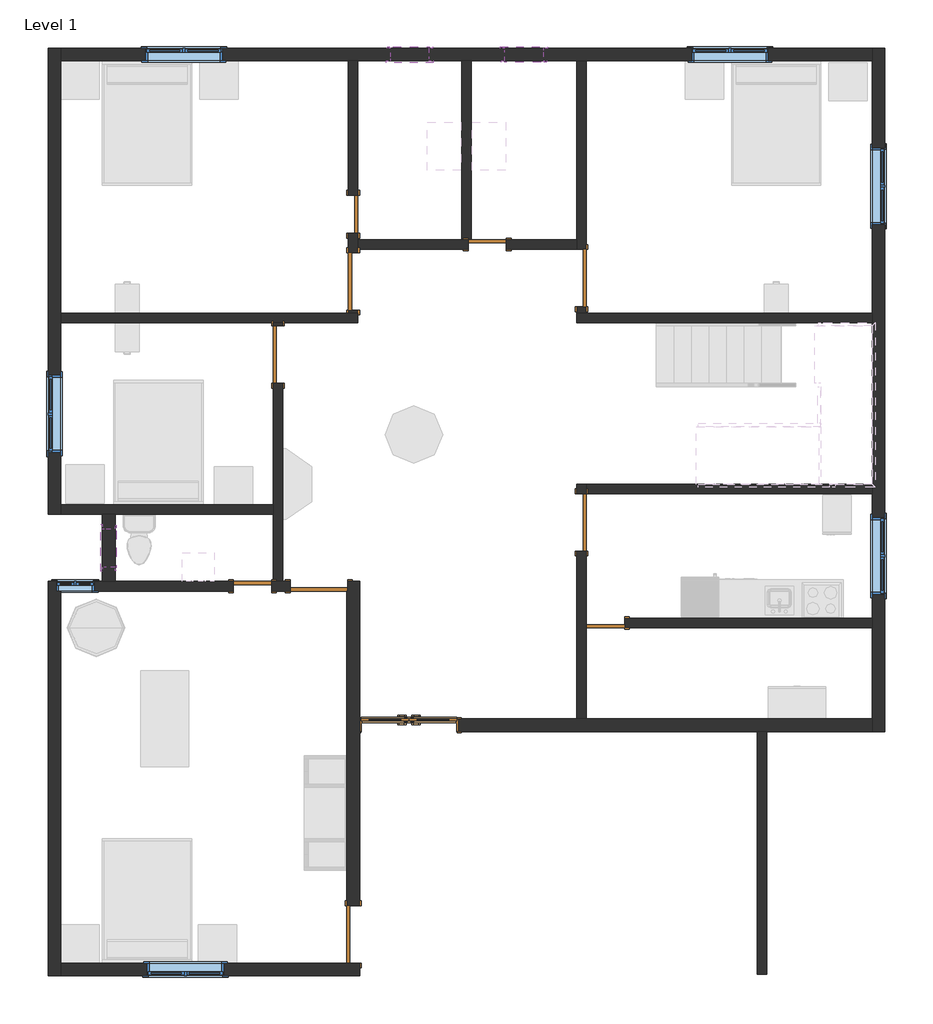
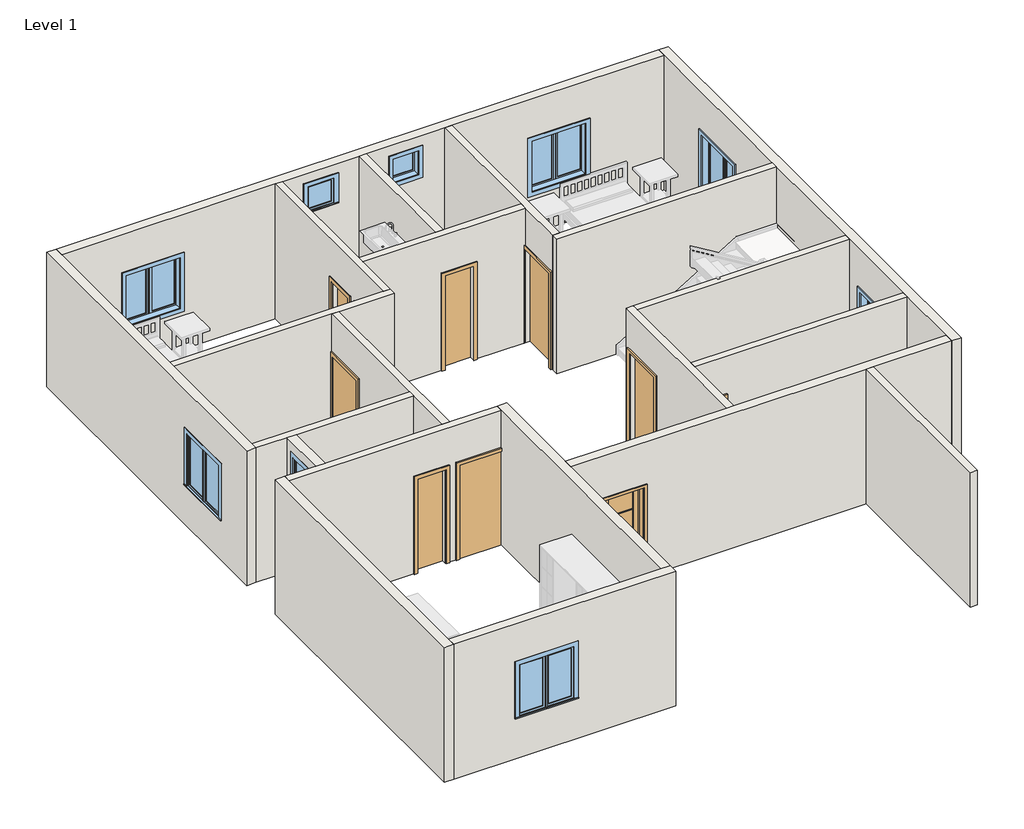
# One storey, part 1 of 2: 21 walls, 11 doors, 10 windows.
"""IFC4 building model written with IfcOpenShell, lengths in millimetres."""

from ifc_helpers import new_model, si_unit, frame, origin, origin_with_axes, place, context, project, spatial, polyline, outline, extrude, faceted_brep, transform, mapped, element, save
from components import door_b03bd389, door_686f89d2, door_719f80de, door_16372e1c, single_flush_door_2_9ea4ff49, single_flush_door_2_5ca4d175, window_0862ab64, casement_dbl_with_trim_window_2_b083d55d, window_e41d21a6

model = new_model("IFC4")

# Units and contexts
model_context = context("Model", 3, world=origin())
ifc_project = project(units=[si_unit("LENGTHUNIT", "METRE", prefix="MILLI")], contexts=[model_context])

# Site, building, storey
site = spatial("IfcSite", under=ifc_project)
building = spatial("IfcBuilding", under=site)
storey = spatial("IfcBuildingStorey", under=building, Name="Level 1", Elevation=0.0)

# Doors
placement = place(None, origin())
door_shape = door_b03bd389(model_context)
element("IfcDoor", 1, ObjectType="Door-Exterior-Double-Full Glass-Wood_Clad : 60\" x 80\"", at=placement, inside=storey, context=model_context, shape_type="MappedRepresentation", body=[
    mapped(door_shape, transform((-10453.8725091, 5079.8899226, 0.0), x_axis=(1.0, 0.0, 0.0), y_axis=(0.0, 1.0, 0.0), z_axis=(0.0, 0.0, 1.0))),
])
door_2_shape = door_686f89d2(model_context)
element("IfcDoor", 2, ObjectType="Single-Flush : 36\" x 84\"", at=placement, inside=storey, context=model_context, shape_type="MappedRepresentation", body=[
    mapped(door_2_shape, transform((-11888.9725091, 7286.5149226, 0.0), x_axis=(1.0, 0.0, 0.0), y_axis=(0.0, 1.0, 0.0), z_axis=(0.0, 0.0, 1.0))),
])
element("IfcDoor", 3, ObjectType="Single-Flush : 36\" x 84\"", at=placement, inside=storey, context=model_context, shape_type="MappedRepresentation", body=[
    mapped(door_2_shape, transform((-7710.6725091, 8302.5149226, 0.0), x_axis=(0.0, 1.0, 0.0), y_axis=(-1.0, 0.0, 0.0), z_axis=(0.0, 0.0, 1.0))),
])
element("IfcDoor", 4, ObjectType="Single-Flush : 36\" x 84\"", at=placement, inside=storey, context=model_context, shape_type="MappedRepresentation", body=[
    mapped(door_2_shape, transform((-11342.8725091, 12137.9149226, 0.0), x_axis=(0.0, -1.0, 0.0), y_axis=(1.0, 0.0, 0.0), z_axis=(0.0, 0.0, 1.0))),
])
door_3_shape = door_719f80de(model_context)
element("IfcDoor", 5, ObjectType="Single-Flush : 36\" x 84\"", at=placement, inside=storey, context=model_context, shape_type="MappedRepresentation", body=[
    mapped(door_3_shape, transform((-11342.8725091, 1749.3149226, 0.0), x_axis=(0.0, -1.0, 0.0), y_axis=(1.0, 0.0, 0.0), z_axis=(0.0, 0.0, 1.0))),
])
door_4_shape = door_16372e1c(model_context)
element("IfcDoor", 6, ObjectType="Single-Flush : 36\" x 84\"", at=placement, inside=storey, context=model_context, shape_type="MappedRepresentation", body=[
    mapped(door_4_shape, transform((-12536.6725091, 10969.5149226, 0.0), x_axis=(0.0, 1.0, 0.0), y_axis=(-1.0, 0.0, 0.0), z_axis=(0.0, 0.0, 1.0))),
])
element("IfcDoor", 7, ObjectType="Single-Flush : 36\" x 84\"", at=placement, inside=storey, context=model_context, shape_type="MappedRepresentation", body=[
    mapped(door_4_shape, transform((-7710.6725091, 12188.7149226, 0.0), x_axis=(0.0, -1.0, 0.0), y_axis=(1.0, 0.0, 0.0), z_axis=(0.0, 0.0, 1.0))),
])
single_flush_door_2_shape = single_flush_door_2_9ea4ff49(model_context)
element("IfcDoor", 8, ObjectType="Single-Flush : door 2", at=placement, inside=storey, context=model_context, shape_type="MappedRepresentation", body=[
    mapped(single_flush_door_2_shape, transform((-7329.6725091, 6702.3149226, 0.0), x_axis=(-1.0, 0.0, 0.0), y_axis=(0.0, -1.0, 0.0), z_axis=(0.0, 0.0, 1.0))),
])
element("IfcDoor", 9, ObjectType="Single-Flush : door 2", at=placement, inside=storey, context=model_context, shape_type="MappedRepresentation", body=[
    mapped(single_flush_door_2_shape, transform((-12943.0725091, 7286.5149226, 0.0), x_axis=(1.0, 0.0, 0.0), y_axis=(0.0, 1.0, 0.0), z_axis=(0.0, 0.0, 1.0))),
])
element("IfcDoor", 10, ObjectType="Single-Flush : door 2", at=placement, inside=storey, context=model_context, shape_type="MappedRepresentation", body=[
    mapped(single_flush_door_2_shape, transform((-11342.8725091, 13204.7149226, 0.0), x_axis=(0.0, -1.0, 0.0), y_axis=(1.0, 0.0, 0.0), z_axis=(0.0, 0.0, 1.0))),
])
single_flush_door_2_2_shape = single_flush_door_2_5ca4d175(model_context)
element("IfcDoor", 11, ObjectType="Single-Flush : door 2", at=placement, inside=storey, context=model_context, shape_type="MappedRepresentation", body=[
    mapped(single_flush_door_2_2_shape, transform((-9209.2725091, 12722.1149226, 0.0), x_axis=(-1.0, 0.0, 0.0), y_axis=(0.0, -1.0, 0.0), z_axis=(0.0, 0.0, 1.0))),
])

# Walls
element("IfcWall", 12, ObjectType="Generic - 8\"", at=placement, inside=storey, context=model_context, shape_type="Brep", body=[
    faceted_brep([(-16194.2725091, 15846.3149226, 0.0), (-16194.2725091, 8429.5149226, 0.0), (-16194.2725091, 8429.5149226, 3048.0), (-16194.2725091, 15846.3149226, 3048.0), (-16194.2725091, 10639.3149226, 2133.6), (-16194.2725091, 9420.1149226, 2133.6), (-16194.2725091, 9420.1149226, 914.4), (-16194.2725091, 10639.3149226, 914.4), (-15991.0725091, 15846.3149226, 0.0), (-15991.0725091, 15846.3149226, 3048.0), (-15991.0725091, 15643.1149226, 3048.0), (-15991.0725091, 11629.9149226, 3048.0), (-15991.0725091, 11477.5149226, 3048.0), (-15991.0725091, 8581.9149226, 3048.0), (-15991.0725091, 8429.5149226, 3048.0), (-15991.0725091, 8429.5149226, 0.0), (-15991.0725091, 8581.9149226, 0.0), (-15991.0725091, 11477.5149226, 0.0), (-15991.0725091, 11629.9149226, 0.0), (-15991.0725091, 15643.1149226, 0.0), (-15991.0725091, 10639.3149226, 2133.6), (-15991.0725091, 10639.3149226, 914.4), (-15991.0725091, 9420.1149226, 914.4), (-15991.0725091, 9420.1149226, 2133.6)], [[[0, 1, 2, 3], [4, 5, 6, 7]], [[8, 9, 10, 11, 12, 13, 14, 15, 16, 17, 18, 19], [20, 21, 22, 23]], [[1, 0, 8, 19, 18, 17, 16, 15]], [[3, 2, 14, 13, 12, 11, 10, 9]], [[0, 3, 9, 8]], [[2, 1, 15, 14]], [[21, 20, 4, 7]], [[22, 21, 7, 6]], [[23, 22, 6, 5]], [[20, 23, 5, 4]]]),
])
element("IfcWall", 13, ObjectType="Generic - 8\"", at=placement, inside=storey, context=model_context, shape_type="Brep", body=[
    faceted_brep([(-15991.0725091, 1088.9149226, 0.0), (-11241.2725091, 1088.9149226, 0.0), (-11241.2725091, 1088.9149226, 3048.0), (-15991.0725091, 1088.9149226, 3048.0), (-14619.4725091, 1088.9149226, 2133.6), (-13400.2725091, 1088.9149226, 2133.6), (-13400.2725091, 1088.9149226, 914.4), (-14619.4725091, 1088.9149226, 914.4), (-15991.0725091, 1292.1149226, 0.0), (-15991.0725091, 1292.1149226, 3048.0), (-11444.4725091, 1292.1149226, 3048.0), (-11241.2725091, 1292.1149226, 3048.0), (-11241.2725091, 1292.1149226, 2133.6), (-11241.2725091, 1292.1149226, 0.0), (-14619.4725091, 1292.1149226, 2133.6), (-14619.4725091, 1292.1149226, 914.4), (-13400.2725091, 1292.1149226, 914.4), (-13400.2725091, 1292.1149226, 2133.6)], [[[0, 1, 2, 3], [4, 5, 6, 7]], [[8, 9, 10, 11, 12, 13], [14, 15, 16, 17]], [[1, 0, 8, 13]], [[3, 2, 11, 10, 9]], [[0, 3, 9, 8]], [[2, 1, 13, 12, 11]], [[15, 14, 4, 7]], [[16, 15, 7, 6]], [[17, 16, 6, 5]], [[14, 17, 5, 4]]]),
])
element("IfcWall", 14, ObjectType="Generic - 8\"", at=placement, inside=storey, context=model_context, shape_type="Brep", body=[
    faceted_brep([(-3087.8725091, 15846.3149226, 0.0), (-15991.0725091, 15846.3149226, 0.0), (-15991.0725091, 15846.3149226, 3048.0), (-3087.8725091, 15846.3149226, 3048.0), (-4738.8725091, 15846.3149226, 2133.6), (-5958.0725091, 15846.3149226, 2133.6), (-5958.0725091, 15846.3149226, 914.4), (-4738.8725091, 15846.3149226, 914.4), (-13425.6725091, 15846.3149226, 2133.6), (-14644.8725091, 15846.3149226, 2133.6), (-14644.8725091, 15846.3149226, 914.4), (-13425.6725091, 15846.3149226, 914.4), (-10745.9725091, 15846.3149226, 2768.6), (-10745.9725091, 15846.3149226, 2159.0), (-10136.3725091, 15846.3149226, 2159.0), (-10136.3725091, 15846.3149226, 2768.6), (-8320.2725091, 15846.3149226, 2768.6), (-8929.8725091, 15846.3149226, 2768.6), (-8929.8725091, 15846.3149226, 2159.0), (-8320.2725091, 15846.3149226, 2159.0), (-3087.8725091, 15643.1149226, 0.0), (-3087.8725091, 15643.1149226, 3048.0), (-7634.4725091, 15643.1149226, 3048.0), (-7786.8725091, 15643.1149226, 3048.0), (-9463.2725091, 15643.1149226, 3048.0), (-9615.6725091, 15643.1149226, 3048.0), (-11266.6725091, 15643.1149226, 3048.0), (-11419.0725091, 15643.1149226, 3048.0), (-15991.0725091, 15643.1149226, 3048.0), (-15991.0725091, 15643.1149226, 0.0), (-11419.0725091, 15643.1149226, 0.0), (-11266.6725091, 15643.1149226, 0.0), (-9615.6725091, 15643.1149226, 0.0), (-9463.2725091, 15643.1149226, 0.0), (-7786.8725091, 15643.1149226, 0.0), (-7634.4725091, 15643.1149226, 0.0), (-4738.8725091, 15643.1149226, 2133.6), (-4738.8725091, 15643.1149226, 914.4), (-5958.0725091, 15643.1149226, 914.4), (-5958.0725091, 15643.1149226, 2133.6), (-13425.6725091, 15643.1149226, 2133.6), (-13425.6725091, 15643.1149226, 914.4), (-14644.8725091, 15643.1149226, 914.4), (-14644.8725091, 15643.1149226, 2133.6), (-10745.9725091, 15643.1149226, 2768.6), (-10136.3725091, 15643.1149226, 2768.6), (-10136.3725091, 15643.1149226, 2159.0), (-10745.9725091, 15643.1149226, 2159.0), (-8320.2725091, 15643.1149226, 2768.6), (-8320.2725091, 15643.1149226, 2159.0), (-8929.8725091, 15643.1149226, 2159.0), (-8929.8725091, 15643.1149226, 2768.6)], [[[0, 1, 2, 3], [4, 5, 6, 7], [8, 9, 10, 11], [12, 13, 14, 15], [16, 17, 18, 19]], [[20, 21, 22, 23, 24, 25, 26, 27, 28, 29, 30, 31, 32, 33, 34, 35], [36, 37, 38, 39], [40, 41, 42, 43], [44, 45, 46, 47], [48, 49, 50, 51]], [[1, 0, 20, 35, 34, 33, 32, 31, 30, 29]], [[3, 2, 28, 27, 26, 25, 24, 23, 22, 21]], [[2, 1, 29, 28]], [[0, 3, 21, 20]], [[37, 36, 4, 7]], [[38, 37, 7, 6]], [[39, 38, 6, 5]], [[36, 39, 5, 4]], [[41, 40, 8, 11]], [[42, 41, 11, 10]], [[43, 42, 10, 9]], [[40, 43, 9, 8]], [[13, 12, 44, 47]], [[14, 13, 47, 46]], [[15, 14, 46, 45]], [[12, 15, 45, 44]], [[49, 48, 16, 19]], [[50, 49, 19, 18]], [[51, 50, 18, 17]], [[48, 51, 17, 16]]]),
])
element("IfcWall", 15, ObjectType="Generic - 8\"", at=placement, inside=storey, context=model_context, shape_type="Brep", body=[
    faceted_brep([(-11444.4725091, 1292.1149226, 3048.0), (-11444.4725091, 7210.3149226, 3048.0), (-11444.4725091, 7362.7149226, 3048.0), (-11444.4725091, 7362.7149226, 2133.6), (-11444.4725091, 7210.3149226, 2133.6), (-11444.4725091, 7210.3149226, 0.0), (-11444.4725091, 2206.5149226, 0.0), (-11444.4725091, 2206.5149226, 2133.6), (-11444.4725091, 1292.1149226, 2133.6), (-11241.2725091, 7362.7149226, 3048.0), (-11241.2725091, 5178.3149226, 3048.0), (-11241.2725091, 4975.1149226, 3048.0), (-11241.2725091, 1292.1149226, 3048.0), (-11241.2725091, 1292.1149226, 2133.6), (-11241.2725091, 2206.5149226, 2133.6), (-11241.2725091, 2206.5149226, 0.0), (-11241.2725091, 7362.7149226, 0.0), (-11431.7725091, 7210.3149226, 0.0), (-11431.7725091, 7362.7149226, 0.0), (-11431.7725091, 7362.7149226, 2133.6), (-11431.7725091, 7210.3149226, 2133.6)], [[[0, 1, 2, 3, 4, 5, 6, 7, 8]], [[9, 10, 11, 12, 13, 14, 15, 16]], [[16, 15, 6, 5, 17, 18]], [[2, 1, 0, 12, 11, 10, 9]], [[2, 9, 16, 18, 19, 3]], [[12, 0, 8, 13]], [[7, 14, 13, 8]], [[14, 7, 6, 15]], [[20, 17, 5, 4]], [[17, 20, 19, 18]], [[19, 20, 4, 3]]]),
])
element("IfcWall", 16, ObjectType="Generic - 8\"", at=placement, inside=storey, context=model_context, shape_type="Brep", body=[
    faceted_brep([(-11241.2725091, 5178.3149226, 3048.0), (-7786.8725091, 5178.3149226, 3048.0), (-7634.4725091, 5178.3149226, 3048.0), (-3087.8725091, 5178.3149226, 3048.0), (-3087.8725091, 5178.3149226, 0.0), (-7634.4725091, 5178.3149226, 0.0), (-7786.8725091, 5178.3149226, 0.0), (-9666.4725091, 5178.3149226, 0.0), (-9666.4725091, 5178.3149226, 2057.4), (-11241.2725091, 5178.3149226, 2057.4), (-3087.8725091, 4975.1149226, 3048.0), (-4764.2725091, 4975.1149226, 3048.0), (-4916.6725091, 4975.1149226, 3048.0), (-11241.2725091, 4975.1149226, 3048.0), (-11241.2725091, 4975.1149226, 2057.4), (-9666.4725091, 4975.1149226, 2057.4), (-9666.4725091, 4975.1149226, 0.0), (-4916.6725091, 4975.1149226, 0.0), (-4764.2725091, 4975.1149226, 0.0), (-3087.8725091, 4975.1149226, 0.0)], [[[0, 1, 2, 3, 4, 5, 6, 7, 8, 9]], [[10, 11, 12, 13, 14, 15, 16, 17, 18, 19]], [[4, 19, 18, 17, 16, 7, 6, 5]], [[3, 2, 1, 0, 13, 12, 11, 10]], [[4, 3, 10, 19]], [[13, 0, 9, 14]], [[15, 8, 7, 16]], [[8, 15, 14, 9]]]),
])
element("IfcWall", 17, ObjectType="Generic - 8\"", at=placement, inside=storey, context=model_context, shape_type="Brep", body=[
    faceted_brep([(-2884.6725091, 4975.1149226, 0.0), (-2884.6725091, 15846.3149226, 0.0), (-2884.6725091, 15846.3149226, 3048.0), (-2884.6725091, 4975.1149226, 3048.0), (-2884.6725091, 7159.5149226, 2133.6), (-2884.6725091, 8378.7149226, 2133.6), (-2884.6725091, 8378.7149226, 914.4), (-2884.6725091, 7159.5149226, 914.4), (-2884.6725091, 13039.6149226, 2133.6), (-2884.6725091, 14258.8149226, 2133.6), (-2884.6725091, 14258.8149226, 914.4), (-2884.6725091, 13039.6149226, 914.4), (-3087.8725091, 4975.1149226, 0.0), (-3087.8725091, 4975.1149226, 3048.0), (-3087.8725091, 5178.3149226, 3048.0), (-3087.8725091, 6626.1149226, 3048.0), (-3087.8725091, 6778.5149226, 3048.0), (-3087.8725091, 8759.7149226, 3048.0), (-3087.8725091, 8912.1149226, 3048.0), (-3087.8725091, 11477.5149226, 3048.0), (-3087.8725091, 11629.9149226, 3048.0), (-3087.8725091, 15643.1149226, 3048.0), (-3087.8725091, 15846.3149226, 3048.0), (-3087.8725091, 15846.3149226, 0.0), (-3087.8725091, 15643.1149226, 0.0), (-3087.8725091, 11629.9149226, 0.0), (-3087.8725091, 11477.5149226, 0.0), (-3087.8725091, 8912.1149226, 0.0), (-3087.8725091, 8759.7149226, 0.0), (-3087.8725091, 6778.5149226, 0.0), (-3087.8725091, 6626.1149226, 0.0), (-3087.8725091, 5178.3149226, 0.0), (-3087.8725091, 7159.5149226, 2133.6), (-3087.8725091, 7159.5149226, 914.4), (-3087.8725091, 8378.7149226, 914.4), (-3087.8725091, 8378.7149226, 2133.6), (-3087.8725091, 13039.6149226, 2133.6), (-3087.8725091, 13039.6149226, 914.4), (-3087.8725091, 14258.8149226, 914.4), (-3087.8725091, 14258.8149226, 2133.6)], [[[0, 1, 2, 3], [4, 5, 6, 7], [8, 9, 10, 11]], [[12, 13, 14, 15, 16, 17, 18, 19, 20, 21, 22, 23, 24, 25, 26, 27, 28, 29, 30, 31], [32, 33, 34, 35], [36, 37, 38, 39]], [[1, 0, 12, 31, 30, 29, 28, 27, 26, 25, 24, 23]], [[3, 2, 22, 21, 20, 19, 18, 17, 16, 15, 14, 13]], [[2, 1, 23, 22]], [[0, 3, 13, 12]], [[33, 32, 4, 7]], [[34, 33, 7, 6]], [[35, 34, 6, 5]], [[32, 35, 5, 4]], [[37, 36, 8, 11]], [[38, 37, 11, 10]], [[39, 38, 10, 9]], [[36, 39, 9, 8]]]),
])
element("IfcWall", 18, ObjectType="Generic - 8\"", at=placement, inside=storey, context=model_context, shape_type="Brep", body=[
    faceted_brep([(-16194.2725091, 7362.7149226, 0.0), (-16194.2725091, 1088.9149226, 0.0), (-16194.2725091, 1088.9149226, 3048.0), (-16194.2725091, 7362.7149226, 3048.0), (-15991.0725091, 1088.9149226, 0.0), (-15991.0725091, 1292.1149226, 0.0), (-15991.0725091, 7210.3149226, 0.0), (-15991.0725091, 7362.7149226, 0.0), (-15991.0725091, 7362.7149226, 914.4), (-15991.0725091, 7210.3149226, 914.4), (-15991.0725091, 7210.3149226, 2133.6), (-15991.0725091, 7362.7149226, 2133.6), (-15991.0725091, 7362.7149226, 3048.0), (-15991.0725091, 7210.3149226, 3048.0), (-15991.0725091, 1292.1149226, 3048.0), (-15991.0725091, 1088.9149226, 3048.0), (-16067.2725091, 7362.7149226, 2133.6), (-16067.2725091, 7362.7149226, 914.4), (-16067.2725091, 7210.3149226, 914.4), (-16067.2725091, 7210.3149226, 2133.6)], [[[0, 1, 2, 3]], [[4, 5, 6, 7, 8, 9, 10, 11, 12, 13, 14, 15]], [[1, 0, 7, 6, 5, 4]], [[3, 2, 15, 14, 13, 12]], [[2, 1, 4, 15]], [[0, 3, 12, 11, 16, 17, 8, 7]], [[18, 19, 10, 9]], [[17, 18, 9, 8]], [[19, 18, 17, 16]], [[19, 16, 11, 10]]]),
])
element("IfcWall", 19, ObjectType="Generic - 8\"", at=placement, inside=storey, context=model_context, shape_type="SweptSolid", body=[
    extrude(outline(polyline([(7362.7149226, 0.0), (7362.7149226, 3048.0), (8429.5149226, 3048.0), (8429.5149226, 0.0), (7362.7149226, 0.0)]), holes=[polyline([(8200.9149226, 2768.6), (7591.3149226, 2768.6), (7591.3149226, 2159.0), (8200.9149226, 2159.0), (8200.9149226, 2768.6)])]), frame((-15330.6725091, 0.0, 0.0), z_axis=(1.0, 0.0, 0.0), x_axis=(0.0, 1.0, 0.0)), (0.0, 0.0, 1.0), 203.2),
])
element("IfcWall", 20, ObjectType="inner wall", at=placement, inside=storey, context=model_context, shape_type="Brep", body=[
    faceted_brep([(-15991.0725091, 11477.5149226, 0.0), (-12612.8725091, 11477.5149226, 0.0), (-12460.4725091, 11477.5149226, 0.0), (-11266.6725091, 11477.5149226, 0.0), (-11266.6725091, 11477.5149226, 3048.0), (-12460.4725091, 11477.5149226, 3048.0), (-12612.8725091, 11477.5149226, 3048.0), (-15991.0725091, 11477.5149226, 3048.0), (-15991.0725091, 11629.9149226, 0.0), (-15991.0725091, 11629.9149226, 3048.0), (-11419.0725091, 11629.9149226, 3048.0), (-11266.6725091, 11629.9149226, 3048.0), (-11266.6725091, 11629.9149226, 0.0), (-11419.0725091, 11629.9149226, 0.0)], [[[0, 1, 2, 3, 4, 5, 6, 7]], [[8, 9, 10, 11, 12, 13]], [[3, 2, 1, 0, 8, 13, 12]], [[7, 6, 5, 4, 11, 10, 9]], [[0, 7, 9, 8]], [[4, 3, 12, 11]]]),
])
element("IfcWall", 21, ObjectType="inner wall", at=placement, inside=storey, context=model_context, shape_type="Brep", body=[
    faceted_brep([(-11266.6725091, 12595.1149226, 0.0), (-11266.6725091, 12645.9149226, 0.0), (-11266.6725091, 12798.3149226, 0.0), (-11266.6725091, 12899.9149226, 0.0), (-11266.6725091, 12899.9149226, 2133.6), (-11266.6725091, 13509.5149226, 2133.6), (-11266.6725091, 13509.5149226, 0.0), (-11266.6725091, 15643.1149226, 0.0), (-11266.6725091, 15643.1149226, 3048.0), (-11266.6725091, 12798.3149226, 3048.0), (-11266.6725091, 12645.9149226, 3048.0), (-11266.6725091, 11629.9149226, 3048.0), (-11266.6725091, 11629.9149226, 0.0), (-11266.6725091, 11680.7149226, 0.0), (-11266.6725091, 11680.7149226, 2133.6), (-11266.6725091, 12595.1149226, 2133.6), (-11419.0725091, 12899.9149226, 2133.6), (-11419.0725091, 12899.9149226, 0.0), (-11419.0725091, 12595.1149226, 0.0), (-11419.0725091, 12595.1149226, 2133.6), (-11419.0725091, 11680.7149226, 2133.6), (-11419.0725091, 11680.7149226, 0.0), (-11419.0725091, 11629.9149226, 0.0), (-11419.0725091, 11629.9149226, 3048.0), (-11419.0725091, 15643.1149226, 3048.0), (-11419.0725091, 15643.1149226, 0.0), (-11419.0725091, 13509.5149226, 0.0), (-11419.0725091, 13509.5149226, 2133.6)], [[[0, 1, 2, 3, 4, 5, 6, 7, 8, 9, 10, 11, 12, 13, 14, 15]], [[16, 17, 18, 19, 20, 21, 22, 23, 24, 25, 26, 27]], [[22, 21, 13, 12]], [[26, 25, 7, 6]], [[18, 17, 3, 2, 1, 0]], [[11, 10, 9, 8, 24, 23]], [[12, 11, 23, 22]], [[8, 7, 25, 24]], [[14, 13, 21, 20]], [[15, 14, 20, 19]], [[0, 15, 19, 18]], [[4, 3, 17, 16]], [[5, 4, 16, 27]], [[6, 5, 27, 26]]]),
])
element("IfcWall", 22, ObjectType="inner wall", at=placement, inside=storey, context=model_context, shape_type="SweptSolid", body=[
    extrude(outline(polyline([(-9615.6725091, 12798.3149226), (-9615.6725091, 15643.1149226), (-9463.2725091, 15643.1149226), (-9463.2725091, 12798.3149226), (-9615.6725091, 12798.3149226)])), origin_with_axes(), (0.0, 0.0, 1.0), 3048.0),
])
element("IfcWall", 23, ObjectType="inner wall", at=placement, inside=storey, context=model_context, shape_type="Brep", body=[
    faceted_brep([(-7786.8725091, 11731.5149226, 2133.6), (-7786.8725091, 11731.5149226, 0.0), (-7786.8725091, 11629.9149226, 0.0), (-7786.8725091, 11629.9149226, 3048.0), (-7786.8725091, 12645.9149226, 3048.0), (-7786.8725091, 12798.3149226, 3048.0), (-7786.8725091, 15643.1149226, 3048.0), (-7786.8725091, 15643.1149226, 0.0), (-7786.8725091, 12798.3149226, 0.0), (-7786.8725091, 12645.9149226, 0.0), (-7786.8725091, 12645.9149226, 2133.6), (-7634.4725091, 11629.9149226, 0.0), (-7634.4725091, 11731.5149226, 0.0), (-7634.4725091, 11731.5149226, 2133.6), (-7634.4725091, 12645.9149226, 2133.6), (-7634.4725091, 12645.9149226, 0.0), (-7634.4725091, 15643.1149226, 0.0), (-7634.4725091, 15643.1149226, 3048.0), (-7634.4725091, 11629.9149226, 3048.0)], [[[0, 1, 2, 3, 4, 5, 6, 7, 8, 9, 10]], [[11, 12, 13, 14, 15, 16, 17, 18]], [[2, 1, 12, 11]], [[9, 8, 7, 16, 15]], [[6, 5, 4, 3, 18, 17]], [[7, 6, 17, 16]], [[3, 2, 11, 18]], [[13, 12, 1, 0]], [[14, 13, 0, 10]], [[15, 14, 10, 9]]]),
])
element("IfcWall", 24, ObjectType="inner wall", at=placement, inside=storey, context=model_context, shape_type="Brep", body=[
    faceted_brep([(-7786.8725091, 11477.5149226, 0.0), (-3087.8725091, 11477.5149226, 0.0), (-3087.8725091, 11477.5149226, 3048.0), (-7786.8725091, 11477.5149226, 3048.0), (-7786.8725091, 11629.9149226, 0.0), (-7786.8725091, 11629.9149226, 3048.0), (-7634.4725091, 11629.9149226, 3048.0), (-3087.8725091, 11629.9149226, 3048.0), (-3087.8725091, 11629.9149226, 0.0), (-7634.4725091, 11629.9149226, 0.0)], [[[0, 1, 2, 3]], [[4, 5, 6, 7, 8, 9]], [[1, 0, 4, 9, 8]], [[3, 2, 7, 6, 5]], [[2, 1, 8, 7]], [[0, 3, 5, 4]]]),
])
element("IfcWall", 25, ObjectType="inner wall", at=placement, inside=storey, context=model_context, shape_type="Brep", body=[
    faceted_brep([(-9514.0725091, 12798.3149226, 2133.6), (-9514.0725091, 12798.3149226, 0.0), (-9615.6725091, 12798.3149226, 0.0), (-11266.6725091, 12798.3149226, 0.0), (-11266.6725091, 12798.3149226, 3048.0), (-9615.6725091, 12798.3149226, 3048.0), (-9463.2725091, 12798.3149226, 3048.0), (-7786.8725091, 12798.3149226, 3048.0), (-7786.8725091, 12798.3149226, 0.0), (-8904.4725091, 12798.3149226, 0.0), (-8904.4725091, 12798.3149226, 2133.6), (-11266.6725091, 12645.9149226, 0.0), (-9514.0725091, 12645.9149226, 0.0), (-9514.0725091, 12645.9149226, 2133.6), (-8904.4725091, 12645.9149226, 2133.6), (-8904.4725091, 12645.9149226, 0.0), (-7786.8725091, 12645.9149226, 0.0), (-7786.8725091, 12645.9149226, 2133.6), (-7786.8725091, 12645.9149226, 3048.0), (-11266.6725091, 12645.9149226, 3048.0)], [[[0, 1, 2, 3, 4, 5, 6, 7, 8, 9, 10]], [[11, 12, 13, 14, 15, 16, 17, 18, 19]], [[9, 8, 16, 15]], [[3, 2, 1, 12, 11]], [[7, 6, 5, 4, 19, 18]], [[8, 7, 18, 17, 16]], [[4, 3, 11, 19]], [[13, 12, 1, 0]], [[14, 13, 0, 10]], [[15, 14, 10, 9]]]),
])
element("IfcWall", 26, ObjectType="inner wall", at=placement, inside=storey, context=model_context, shape_type="Brep", body=[
    faceted_brep([(-15991.0725091, 8429.5149226, 0.0), (-15330.6725091, 8429.5149226, 0.0), (-15127.4725091, 8429.5149226, 0.0), (-12612.8725091, 8429.5149226, 0.0), (-12612.8725091, 8429.5149226, 3048.0), (-15127.4725091, 8429.5149226, 3048.0), (-15330.6725091, 8429.5149226, 3048.0), (-15991.0725091, 8429.5149226, 3048.0), (-15991.0725091, 8581.9149226, 0.0), (-15991.0725091, 8581.9149226, 3048.0), (-12612.8725091, 8581.9149226, 3048.0), (-12612.8725091, 8581.9149226, 0.0)], [[[0, 1, 2, 3, 4, 5, 6, 7]], [[8, 9, 10, 11]], [[3, 2, 1, 0, 8, 11]], [[7, 6, 5, 4, 10, 9]], [[4, 3, 11, 10]], [[0, 7, 9, 8]]]),
])
element("IfcWall", 27, ObjectType="inner wall", at=placement, inside=storey, context=model_context, shape_type="Brep", body=[
    faceted_brep([(-15991.0725091, 7362.7149226, 3048.0), (-15330.6725091, 7362.7149226, 3048.0), (-15127.4725091, 7362.7149226, 3048.0), (-12612.8725091, 7362.7149226, 3048.0), (-12460.4725091, 7362.7149226, 3048.0), (-11444.4725091, 7362.7149226, 3048.0), (-11444.4725091, 7362.7149226, 2133.6), (-12346.1725091, 7362.7149226, 2133.6), (-12346.1725091, 7362.7149226, 0.0), (-12460.4725091, 7362.7149226, 0.0), (-12612.8725091, 7362.7149226, 0.0), (-12638.2725091, 7362.7149226, 0.0), (-12638.2725091, 7362.7149226, 2133.6), (-13247.8725091, 7362.7149226, 2133.6), (-13247.8725091, 7362.7149226, 0.0), (-15127.4725091, 7362.7149226, 0.0), (-15330.6725091, 7362.7149226, 0.0), (-15991.0725091, 7362.7149226, 0.0), (-15991.0725091, 7362.7149226, 914.4), (-15457.6725091, 7362.7149226, 914.4), (-15457.6725091, 7362.7149226, 2133.6), (-15991.0725091, 7362.7149226, 2133.6), (-11444.4725091, 7210.3149226, 3048.0), (-15991.0725091, 7210.3149226, 3048.0), (-15991.0725091, 7210.3149226, 2133.6), (-15457.6725091, 7210.3149226, 2133.6), (-15457.6725091, 7210.3149226, 914.4), (-15991.0725091, 7210.3149226, 914.4), (-15991.0725091, 7210.3149226, 0.0), (-13247.8725091, 7210.3149226, 0.0), (-13247.8725091, 7210.3149226, 2133.6), (-12638.2725091, 7210.3149226, 2133.6), (-12638.2725091, 7210.3149226, 0.0), (-12346.1725091, 7210.3149226, 0.0), (-12346.1725091, 7210.3149226, 2133.6), (-11444.4725091, 7210.3149226, 2133.6)], [[[0, 1, 2, 3, 4, 5, 6, 7, 8, 9, 10, 11, 12, 13, 14, 15, 16, 17, 18, 19, 20, 21]], [[22, 23, 24, 25, 26, 27, 28, 29, 30, 31, 32, 33, 34, 35]], [[32, 11, 10, 9, 8, 33]], [[14, 29, 28, 17, 16, 15]], [[5, 4, 3, 2, 1, 0, 23, 22]], [[5, 22, 35, 6]], [[12, 11, 32, 31]], [[13, 12, 31, 30]], [[14, 13, 30, 29]], [[34, 7, 6, 35]], [[7, 34, 33, 8]], [[17, 28, 27, 18]], [[23, 0, 21, 24]], [[25, 20, 19, 26]], [[26, 19, 18, 27]], [[20, 25, 24, 21]]]),
])
element("IfcWall", 28, ObjectType="inner wall", at=placement, inside=storey, context=model_context, shape_type="Brep", body=[
    faceted_brep([(-12612.8725091, 11477.5149226, 0.0), (-12612.8725091, 11426.7149226, 0.0), (-12612.8725091, 11426.7149226, 2133.6), (-12612.8725091, 10512.3149226, 2133.6), (-12612.8725091, 10512.3149226, 0.0), (-12612.8725091, 8581.9149226, 0.0), (-12612.8725091, 8429.5149226, 0.0), (-12612.8725091, 7362.7149226, 0.0), (-12612.8725091, 7362.7149226, 3048.0), (-12612.8725091, 8429.5149226, 3048.0), (-12612.8725091, 8581.9149226, 3048.0), (-12612.8725091, 11477.5149226, 3048.0), (-12460.4725091, 11426.7149226, 2133.6), (-12460.4725091, 11426.7149226, 0.0), (-12460.4725091, 11477.5149226, 0.0), (-12460.4725091, 11477.5149226, 3048.0), (-12460.4725091, 7362.7149226, 3048.0), (-12460.4725091, 7362.7149226, 0.0), (-12460.4725091, 10512.3149226, 0.0), (-12460.4725091, 10512.3149226, 2133.6)], [[[0, 1, 2, 3, 4, 5, 6, 7, 8, 9, 10, 11]], [[12, 13, 14, 15, 16, 17, 18, 19]], [[18, 17, 7, 6, 5, 4]], [[14, 13, 1, 0]], [[11, 10, 9, 8, 16, 15]], [[0, 11, 15, 14]], [[8, 7, 17, 16]], [[2, 1, 13, 12]], [[3, 2, 12, 19]], [[4, 3, 19, 18]]]),
])
element("IfcWall", 29, ObjectType="inner wall", at=placement, inside=storey, context=model_context, shape_type="Brep", body=[
    faceted_brep([(-7634.4725091, 8759.7149226, 2133.6), (-7634.4725091, 8759.7149226, 0.0), (-7634.4725091, 8912.1149226, 0.0), (-7634.4725091, 8912.1149226, 3048.0), (-7634.4725091, 8759.7149226, 3048.0), (-7634.4725091, 6778.5149226, 3048.0), (-7634.4725091, 6626.1149226, 3048.0), (-7634.4725091, 5178.3149226, 3048.0), (-7634.4725091, 5178.3149226, 0.0), (-7634.4725091, 7845.3149226, 0.0), (-7634.4725091, 7845.3149226, 2133.6), (-7786.8725091, 8912.1149226, 0.0), (-7786.8725091, 8759.7149226, 0.0), (-7786.8725091, 8759.7149226, 2133.6), (-7786.8725091, 7845.3149226, 2133.6), (-7786.8725091, 7845.3149226, 0.0), (-7786.8725091, 5178.3149226, 0.0), (-7786.8725091, 5178.3149226, 3048.0), (-7786.8725091, 8912.1149226, 3048.0)], [[[0, 1, 2, 3, 4, 5, 6, 7, 8, 9, 10]], [[11, 12, 13, 14, 15, 16, 17, 18]], [[9, 8, 16, 15]], [[2, 1, 12, 11]], [[7, 6, 5, 4, 3, 18, 17]], [[8, 7, 17, 16]], [[3, 2, 11, 18]], [[13, 12, 1, 0]], [[14, 13, 0, 10]], [[15, 14, 10, 9]]]),
])
element("IfcWall", 30, ObjectType="inner wall", at=placement, inside=storey, context=model_context, shape_type="SweptSolid", body=[
    extrude(outline(polyline([(-3087.8725091, 8759.7149226), (-7634.4725091, 8759.7149226), (-7634.4725091, 8912.1149226), (-3087.8725091, 8912.1149226), (-3087.8725091, 8759.7149226)])), origin_with_axes(), (0.0, 0.0, 1.0), 3048.0),
])
element("IfcWall", 31, ObjectType="inner wall", at=placement, inside=storey, context=model_context, shape_type="SweptSolid", body=[
    extrude(outline(polyline([(3048.0, -3087.8725091), (3048.0, -7634.4725091), (2133.6, -7634.4725091), (2133.6, -7024.8725091), (0.0, -7024.8725091), (0.0, -3087.8725091), (3048.0, -3087.8725091)])), frame((0.0, 6626.1149226, 0.0), z_axis=(0.0, 1.0, 0.0), x_axis=(0.0, 0.0, 1.0)), (0.0, 0.0, 1.0), 152.4),
])
element("IfcWall", 32, ObjectType="inner wall", at=placement, inside=storey, context=model_context, shape_type="SweptSolid", body=[
    extrude(outline(polyline([(-4916.6725091, 1114.3149226), (-4916.6725091, 4975.1149226), (-4764.2725091, 4975.1149226), (-4764.2725091, 1114.3149226), (-4916.6725091, 1114.3149226)])), origin_with_axes(), (0.0, 0.0, 1.0), 3048.0),
])

# Windows
window_shape = window_0862ab64(model_context)
element("IfcWindow", 33, ObjectType="Casement Dbl with Trim : 48\" x 48\"", at=placement, inside=storey, context=model_context, shape_type="MappedRepresentation", body=[
    mapped(window_shape, transform((-14009.8725091, 1209.5649226, 0.0), x_axis=(-1.0, 0.0, 0.0), y_axis=(0.0, -1.0, 0.0), z_axis=(0.0, 0.0, 1.0))),
])
element("IfcWindow", 34, ObjectType="Casement Dbl with Trim : 48\" x 48\"", at=placement, inside=storey, context=model_context, shape_type="MappedRepresentation", body=[
    mapped(window_shape, transform((-3005.3225091, 7769.1149226, 0.0), x_axis=(0.0, -1.0, 0.0), y_axis=(1.0, 0.0, 0.0), z_axis=(0.0, 0.0, 1.0))),
])
element("IfcWindow", 35, ObjectType="Casement Dbl with Trim : 48\" x 48\"", at=placement, inside=storey, context=model_context, shape_type="MappedRepresentation", body=[
    mapped(window_shape, transform((-3005.3225091, 13649.2149226, 0.0), x_axis=(0.0, -1.0, 0.0), y_axis=(1.0, 0.0, 0.0), z_axis=(0.0, 0.0, 1.0))),
])
element("IfcWindow", 36, ObjectType="Casement Dbl with Trim : 48\" x 48\"", at=placement, inside=storey, context=model_context, shape_type="MappedRepresentation", body=[
    mapped(window_shape, transform((-5348.4725091, 15725.6649226, 0.0), x_axis=(1.0, 0.0, 0.0), y_axis=(0.0, 1.0, 0.0), z_axis=(0.0, 0.0, 1.0))),
])
element("IfcWindow", 37, ObjectType="Casement Dbl with Trim : 48\" x 48\"", at=placement, inside=storey, context=model_context, shape_type="MappedRepresentation", body=[
    mapped(window_shape, transform((-14035.2725091, 15725.6649226, 0.0), x_axis=(1.0, 0.0, 0.0), y_axis=(0.0, 1.0, 0.0), z_axis=(0.0, 0.0, 1.0))),
])
element("IfcWindow", 38, ObjectType="Casement Dbl with Trim : 48\" x 48\"", at=placement, inside=storey, context=model_context, shape_type="MappedRepresentation", body=[
    mapped(window_shape, transform((-16073.6225091, 10029.7149226, 0.0), x_axis=(0.0, 1.0, 0.0), y_axis=(-1.0, 0.0, 0.0), z_axis=(0.0, 0.0, 1.0))),
])
casement_dbl_with_trim_window_2_shape = casement_dbl_with_trim_window_2_b083d55d(model_context)
element("IfcWindow", 39, ObjectType="Casement Dbl with Trim : window 2", at=placement, inside=storey, context=model_context, shape_type="MappedRepresentation", body=[
    mapped(casement_dbl_with_trim_window_2_shape, transform((-15762.4725091, 7267.4649226, 0.0), x_axis=(1.0, 0.0, 0.0), y_axis=(0.0, 1.0, 0.0), z_axis=(0.0, 0.0, 1.0))),
])
window_2_shape = window_e41d21a6(model_context)
element("IfcWindow", 40, ObjectType="Transom with Trim : 24\" x 24\"", at=placement, inside=storey, context=model_context, shape_type="MappedRepresentation", body=[
    mapped(window_2_shape, transform((-15229.0725091, 7934.2149226, 0.0), x_axis=(0.0, 1.0, 0.0), y_axis=(-1.0, 0.0, 0.0), z_axis=(0.0, 0.0, 1.0))),
])
element("IfcWindow", 41, ObjectType="Transom with Trim : 24\" x 24\"", at=placement, inside=storey, context=model_context, shape_type="MappedRepresentation", body=[
    mapped(window_2_shape, transform((-10479.2725091, 15744.7149226, 0.0), x_axis=(-1.0, 0.0, 0.0), y_axis=(0.0, -1.0, 0.0), z_axis=(0.0, 0.0, 1.0))),
])
element("IfcWindow", 42, ObjectType="Transom with Trim : 24\" x 24\"", at=placement, inside=storey, context=model_context, shape_type="MappedRepresentation", body=[
    mapped(window_2_shape, transform((-8586.9725091, 15744.7149226, 0.0), x_axis=(1.0, 0.0, 0.0), y_axis=(0.0, 1.0, 0.0), z_axis=(0.0, 0.0, 1.0))),
])

save(model, "model.ifc")

# Revit data of these elements
# Type "Door-Exterior-Double-Full Glass-Wood_Clad : 60\" x 80\""
#   Type Mark = "9"
#   Assembly Code = "B2030100"
#   Analytic Construction = "French door, wood frame with double glass"
#   Top Rail = 0' - 4 11/16"
#   Threshold Offset [instance default] = 0' - 0 1/2"
#   Thickness = 0' - 1 3/8"
#   Thermal Resistance (R) = 1.9158 (h·ft²·°F)/BTU
#   Swing Angle [instance default] = 90.00°
#   Stiles = 0' - 4 3/4"
#   Rough Width = 5' - 2"
#   Rough Height = 6' - 9"
#   Panel Width = 2' - 6"
#   Door Offset [instance default] = 0' - 0"
#   Height = 6' - 8"
#   Width = 5' - 0"
#   Heat Transfer Coefficient (U) = 0.5220 BTU/(h·ft²·°F)
#   Bottom Rail = 0' - 9 1/8"
#   Exterior Trim [instance default] = yes
#   Threshold [instance default] = yes
#   Show Grill [instance default] = yes
#   Function = 1
#   Trim Material = Cherry
#   Threshold Material = Cherry
#   Panel Material = Cherry
#   Glazing = Glass
#   Frame Material = Cherry
#   Door Handle Material = Aluminum
#   Visual Light Transmittance = 0
#   Solar Heat Gain Coefficient = 0
#   Wall Closure = (empty or 0)
#   Construction Type = (empty or 0)
# Type "Single-Flush : 36\" x 84\""
#   Type Mark = "1"
#   Construction Type Id = "MDOOR"
#   Assembly Code = "C1020"
#   Analytic Construction = "Metal"
#   Thickness = 0' - 2"
#   Heat Transfer Coefficient (U) = 0.651978 BTU/(h·ft²·°F)
#   Height = 7' - 0"
#   Trim Projection Ext = 0' - 1"
#   Trim Projection Int = 0' - 1"
#   Trim Width = 0' - 3"
#   Width = 3' - 0"
#   Define Thermal Properties by = 1
#   Door Material = Door - Panel
#   Frame Material = Door - Frame
#   Visual Light Transmittance = 0
#   Solar Heat Gain Coefficient = 0
#   Function = (empty or 0)
#   Wall Closure = (empty or 0)
# Type "Single-Flush : door 2"
#   Type Mark = "8"
#   Construction Type Id = "MDOOR"
#   Assembly Code = "C1020"
#   Analytic Construction = "Metal"
#   Thickness = 0' - 2"
#   Heat Transfer Coefficient (U) = 0.651978 BTU/(h·ft²·°F)
#   Height = 7' - 0"
#   Trim Projection Ext = 0' - 1"
#   Trim Projection Int = 0' - 1"
#   Trim Width = 0' - 3"
#   Width = 2' - 0"
#   Define Thermal Properties by = 1
#   Door Material = Door - Panel
#   Frame Material = Door - Frame
#   Visual Light Transmittance = 0
#   Solar Heat Gain Coefficient = 0
#   Function = (empty or 0)
#   Wall Closure = (empty or 0)
# Type "Generic - 8\""
#   Assembly Code = "B2010"
#   Layers, outside or top first: 0' - 8" no material (function 1)
# Type "inner wall"
#   Assembly Code = "B2010"
#   Layers, outside or top first: 0' - 6" no material (function 1)
# Type "Casement Dbl with Trim : 48\" x 48\""
#   Type Mark = "10"
#   Construction Type Id = "GSP4R"
#   Assembly Code = "B2020100"
#   Analytic Construction = "1/8 in Pilkington single glazing"
#   Visual Light Transmittance = 0.9
#   Solar Heat Gain Coefficient = 0.78
#   Heat Transfer Coefficient (U) = 0.6496 BTU/(h·ft²·°F)
#   Height = 4' - 0"
#   Default Sill Height = 3' - 0"
#   Trim Projection - Ext. = 0' - 0 1/2"
#   Trim Projection - Int. = 0' - 0 3/4"
#   Trim Width - Exterior = 0' - 3 1/2"
#   Trim Width - Interior = 0' - 3 1/2"
#   Width = 4' - 0"
#   Window Inset = 0' - 0 3/4"
#   Define Thermal Properties by = 1
#   Glass Pane Material = Glass
#   Sash Material = Sash
#   Trim Exterior Material = Trim
#   Trim Interior Material = Trim
#   Wall Closure = (empty or 0)
# Type "Casement Dbl with Trim : window 2"
#   Type Mark = "13"
#   Construction Type Id = "GSP4R"
#   Assembly Code = "B2020100"
#   Analytic Construction = "1/8 in Pilkington single glazing"
#   Visual Light Transmittance = 0.9
#   Solar Heat Gain Coefficient = 0.78
#   Heat Transfer Coefficient (U) = 0.6496 BTU/(h·ft²·°F)
#   Height = 4' - 0"
#   Default Sill Height = 3' - 0"
#   Trim Projection - Ext. = 0' - 0 1/2"
#   Trim Projection - Int. = 0' - 0 3/4"
#   Trim Width - Exterior = 0' - 3 1/2"
#   Trim Width - Interior = 0' - 3 1/2"
#   Width = 2' - 0"
#   Window Inset = 0' - 0 3/4"
#   Define Thermal Properties by = 1
#   Glass Pane Material = Glass
#   Sash Material = Sash
#   Trim Exterior Material = Trim
#   Trim Interior Material = Trim
#   Wall Closure = (empty or 0)
# Type "Transom with Trim : 24\" x 24\""
#   Type Mark = "14"
#   Construction Type Id = "GSP4R"
#   Assembly Code = "B2020100"
#   Analytic Construction = "1/8 in Pilkington single glazing"
#   Visual Light Transmittance = 0.9
#   Solar Heat Gain Coefficient = 0.78
#   Heat Transfer Coefficient (U) = 0.6496 BTU/(h·ft²·°F)
#   Height = 2' - 0"
#   Default Sill Height = 7' - 1"
#   Trim Projection - Ext. = 0' - 0 1/2"
#   Trim Projection - Int. = 0' - 0 3/4"
#   Trim Width - Exterior = 0' - 3 1/2"
#   Trim Width - Interior = 0' - 3 1/2"
#   Width = 2' - 0"
#   Window Inset = 0' - 0 3/4"
#   Define Thermal Properties by = 1
#   Glass Pane Material = Glass
#   Sash Material = Sash
#   Trim Exterior Material = Trim
#   Trim Interior Material = Trim
#   Wall Closure = (empty or 0)
# Element 1 (IfcDoor, "Door-Exterior-Double-Full Glass-Wood_Clad : 60\" x 80\"")
#   Threshold Offset = 0' - 0 1/2"
#   Swing Angle = 90.00°
#   Door Offset = 0' - 0"
#   Threshold = yes
#   Show Grill = yes
#   Exterior Trim = yes
#   Phase Created = New Construction
#   Materials on its faces: "Cherry", "Aluminum", "Glass"
# Elements 2, 3, 4, 5, 6, 7 (IfcDoor, "Single-Flush : 36\" x 84\"")
#   Phase Created = New Construction
#   Materials on its faces: "Door - Frame", "Door - Panel"
# Elements 8, 9, 10, 11 (IfcDoor, "Single-Flush : door 2")
#   Phase Created = New Construction
#   Materials on its faces: "Door - Frame", "Door - Panel"
# Elements 12, 13, 14, 15, 16, 17, 18, 19 (IfcWall, "Generic - 8\"")
#   Top Offset = 0' - 0"
#   Base Offset = 0' - 0"
#   Unconnected Height = 10' - 0"
#   wall height = 10' - 0"
#   Phase Created = New Construction
#   Base Constraint = Level 1
#   Materials on its faces: "Default Wall"
# Elements 20, 21, 22, 23, 24, 25, 26, 27, 28, 29, 30, 31, 32 (IfcWall, "inner wall")
#   Top Offset = 0' - 0"
#   Base Offset = 0' - 0"
#   Unconnected Height = 10' - 0"
#   wall height = 10' - 0"
#   Phase Created = New Construction
#   Base Constraint = Level 1
#   Materials on its faces: "Default Wall"
# Element 33 (IfcWindow, "Casement Dbl with Trim : 48\" x 48\"")
#   Mark = "1"
#   Phase Created = New Construction
#   Materials on its faces: "Sash", "Trim", "Glass"
# Element 34 (IfcWindow, "Casement Dbl with Trim : 48\" x 48\"")
#   Mark = "2"
#   Phase Created = New Construction
#   Materials on its faces: "Sash", "Trim", "Glass"
# Element 35 (IfcWindow, "Casement Dbl with Trim : 48\" x 48\"")
#   Mark = "3"
#   Phase Created = New Construction
#   Materials on its faces: "Sash", "Trim", "Glass"
# Element 36 (IfcWindow, "Casement Dbl with Trim : 48\" x 48\"")
#   Mark = "4"
#   Phase Created = New Construction
#   Materials on its faces: "Sash", "Trim", "Glass"
# Element 37 (IfcWindow, "Casement Dbl with Trim : 48\" x 48\"")
#   Mark = "5"
#   Phase Created = New Construction
#   Materials on its faces: "Sash", "Trim", "Glass"
# Element 38 (IfcWindow, "Casement Dbl with Trim : 48\" x 48\"")
#   Mark = "8"
#   Phase Created = New Construction
#   Materials on its faces: "Sash", "Trim", "Glass"
# Element 39 (IfcWindow, "Casement Dbl with Trim : window 2")
#   Mark = "7"
#   Phase Created = New Construction
#   Materials on its faces: "Sash", "Trim", "Glass"
# Element 40 (IfcWindow, "Transom with Trim : 24\" x 24\"")
#   Mark = "9"
#   Phase Created = New Construction
#   Materials on its faces: "Sash", "Trim", "Glass"
# Element 41 (IfcWindow, "Transom with Trim : 24\" x 24\"")
#   Mark = "10"
#   Phase Created = New Construction
#   Materials on its faces: "Sash", "Trim", "Glass"
# Element 42 (IfcWindow, "Transom with Trim : 24\" x 24\"")
#   Mark = "11"
#   Phase Created = New Construction
#   Materials on its faces: "Sash", "Trim", "Glass"
# Materials
#   "Cherry": class "Wood", colour RGB 226 177 128, transparency 0, Description = "Prunus Serotina", Cost = 0
#   "Glass": class "Glass", colour RGB 0 128 192, transparency 0.75, Description = "Soda Lime Glass", Cost = 0
#   "Aluminum": class "Metal", colour RGB 247 247 247, transparency 0, Description = "Aluminum 6061", Cost = 0
#   "Door - Panel": class "Wood", colour RGB 210 159 95, transparency 0
#   "Door - Frame": colour RGB 118 70 51, transparency 0
#   "Sash": class "Wood", colour RGB 224 178 126, transparency 0
#   "Trim": class "Wood", colour RGB 224 178 126, transparency 0
#   "Default Wall": colour RGB 128 128 128, transparency 0
# Room at (-13392.982, 13781.747) mm, phase "New Construction", upper level "Level 1", upper offset 10' - 0", lower offset 0' - 0"
#   Number = "1"
#   Name = "BED ROOM 1"
# Room at (-14447.518, 10174.124) mm, phase "New Construction", upper level "Level 1", upper offset 10' - 0", lower offset 0' - 0"
#   Number = "2"
#   Name = "BED ROOM 3"
# Room at (-13975.752, 8203.807) mm, phase "New Construction", upper level "Level 1", upper offset 10' - 0", lower offset 0' - 0"
#   Number = "3"
#   Name = "WC+BATH"
# Room at (-13392.982, 4540.682) mm, phase "New Construction", upper level "Level 1", upper offset 10' - 0", lower offset 0' - 0"
#   Number = "4"
#   Name = "GUEST ROOM"
# Room at (-7676.288, 3278.527) mm, phase "New Construction", upper level "Level 1", upper offset 10' - 0", lower offset 0' - 0"
#   Number = "5"
#   Name = "VERANDA AREA"
# Room at (-3929.91, 3278.527) mm, phase "New Construction", upper level "Level 1", upper offset 10' - 0", lower offset 0' - 0"
#   Number = "6"
#   Name = "PORCH"
# Room at (-5345.208, 6261.241) mm, phase "New Construction", upper level "Level 1", upper offset 10' - 0", lower offset 0' - 0"
#   Number = "7"
#   Name = "STORE ROOM"
# Room at (-5345.208, 8203.807) mm, phase "New Construction", upper level "Level 1", upper offset 10' - 0", lower offset 0' - 0"
#   Number = "8"
#   Name = "KITCHEN"
# Room at (-10645.639, 14364.517) mm, phase "New Construction", upper level "Level 1", upper offset 10' - 0", lower offset 0' - 0"
#   Number = "11"
#   Name = "WC+BATH"
# Room at (-9826.934, 9312.787) mm, phase "New Construction", upper level "Level 1", upper offset 10' - 0", lower offset 0' - 0"
#   Number = "12"
# Room at (-8869.578, 14364.517) mm, phase "New Construction", upper level "Level 1", upper offset 10' - 0", lower offset 0' - 0"
#   Number = "10"
#   Name = "WC+BATH"
# Room at (-5345.208, 13226.728) mm, phase "New Construction", upper level "Level 1", upper offset 10' - 0", lower offset 0' - 0"
#   Number = "9"
#   Name = "BED ROOM 2"
